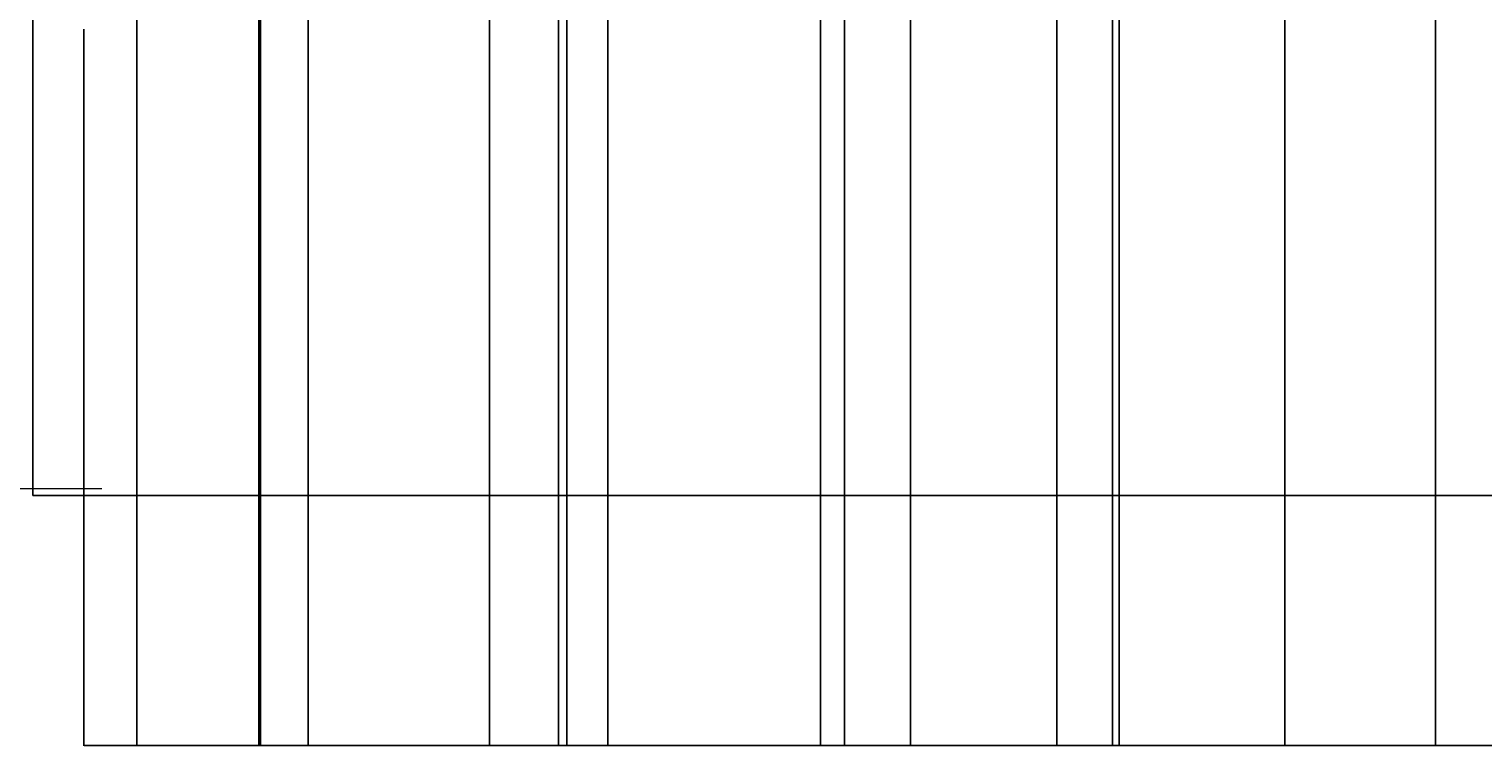
# Model space of a CAD drawing. Units: inches. Extents: x 154617 to 156384, y 250671 to 252576.
# Tile 2 of 6: x 155207 to 155945, y 250671 to 251035. Entities that reach past the tile are written whole.
import ezdxf

# ---------------------------------------------------------------- set-up
doc = ezdxf.new("R2010")
doc.units = ezdxf.units.IN
for name, color, linetype, lineweight in [('A-ANNO-DIMS', 2, 'Continuous', 18), ('C-ANNO-BRKL', 7, 'Continuous', 18), ('C-ROAD', 7, 'Continuous', 25)]:
    doc.layers.add(name, color=color, linetype=linetype, lineweight=lineweight)
doc.styles.get("Standard").update_dxf_attribs({"font": 'arial.ttf'})
doc.dimstyles.get("Standard").update_dxf_attribs({"dimtxt": 0.18, "dimasz": 0.18, "dimexe": 0.18, "dimexo": 0.0625, "dimgap": 0.09, "dimtad": 0, "dimtih": 1, "dimtoh": 1, "dimdec": 4, "dimzin": 0, "dimdsep": 46, "dimtxsty": 'Standard', "dimcen": 0.09, "dimadec": 0, "dimazin": 0, "dimtfac": 1, "dimtdec": 4, "dimtofl": 0, "dimtmove": 0, "dimatfit": 3, "dimfxl": 1, "dimtolj": 1, "dimtzin": 0, "dimarcsym": 0})

# ---------------------------------------------------------------- blocks, each defined once
blk = doc.blocks.new('ROAD-BREAK')
for p, q in [((319.88, 114.19), (261.89, 43.25)), ((319.88, 0), (319.88, 114.19)), ((261.89, 43.25), (0, 43.25)), ((344.19, 43.25), (319.88, 0)), ((540.36, 43.25), (344.19, 43.25))]:
    blk.add_line(p, q)
blk = doc.blocks.new('*D19')
at = {"layer": 'A-ANNO-DIMS', "color": 0, "lineweight": -2, "transparency": 16777216}
for p, q in [((155235.1, 251034.96), (155235.1, 250671.2)), ((156296.1, 251034.96), (156296.1, 250671.2)), ((155235.28, 250671.38), (155765.26, 250671.38)), ((156295.92, 250671.38), (155765.93, 250671.38))]:
    blk.add_line(p, q, dxfattribs=at)
at = {"layer": 'A-ANNO-DIMS', "color": 0, "transparency": 16777216}
for points in [[(155235.28, 250671.41), (155235.28, 250671.35), (155235.1, 250671.38)], [(156295.92, 250671.41), (156295.92, 250671.35), (156296.1, 250671.38)]]:
    blk.add_solid(points, dxfattribs=at)
at = {"layer": 'Defpoints', "color": 0, "transparency": 16777216}
for p in [(155235.1, 251035.03), (156296.1, 251035.03), (156296.1, 250671.38)]:
    blk.add_point(p, dxfattribs=at)
at = {"layer": 'A-ANNO-DIMS', "color": 0, "transparency": 16777216, "insert": (155765.6, 250671.38), "char_height": 0.18, "attachment_point": 5}
blk.add_mtext('\\A1;1061', dxfattribs=at)
blk = doc.blocks.new('*D24')
at = {"layer": 'A-ANNO-DIMS', "color": 0, "lineweight": -2, "transparency": 16777216}
for p, q in [((156296.16, 251035.03), (156383.38, 251035.03)), ((156383.2, 251034.85), (156383.2, 250916.83)), ((156383.2, 250798.45), (156383.2, 250916.46)), ((155209.3, 250798.27), (156383.38, 250798.27))]:
    blk.add_line(p, q, dxfattribs=at)
at = {"layer": 'A-ANNO-DIMS', "color": 0, "transparency": 16777216}
for points in [[(156383.17, 251034.85), (156383.23, 251034.85), (156383.2, 251035.03)], [(156383.17, 250798.45), (156383.23, 250798.45), (156383.2, 250798.27)]]:
    blk.add_solid(points, dxfattribs=at)
at = {"layer": 'Defpoints', "color": 0, "transparency": 16777216}
for p in [(156296.1, 251035.03), (156383.2, 251035.03), (155209.24, 250798.27)]:
    blk.add_point(p, dxfattribs=at)
at = {"layer": 'A-ANNO-DIMS', "color": 0, "transparency": 16777216, "insert": (156383.2, 250916.65), "char_height": 0.18, "attachment_point": 5}
blk.add_mtext('\\A1;236.76', dxfattribs=at)
blk = doc.blocks.new('*D36')
at = {"layer": 'A-ANNO-DIMS', "color": 0, "lineweight": -2, "transparency": 16777216}
for p, q in [((155324.84, 251443.46), (155324.84, 250671.2)), ((155475.98, 251443.46), (155475.98, 250671.2)), ((155325.02, 250671.38), (155399.96, 250671.38)), ((155475.8, 250671.38), (155400.87, 250671.38))]:
    blk.add_line(p, q, dxfattribs=at)
at = {"layer": 'A-ANNO-DIMS', "color": 0, "transparency": 16777216}
for points in [[(155325.02, 250671.41), (155325.02, 250671.35), (155324.84, 250671.38)], [(155475.8, 250671.41), (155475.8, 250671.35), (155475.98, 250671.38)]]:
    blk.add_solid(points, dxfattribs=at)
at = {"layer": 'Defpoints', "color": 0, "transparency": 16777216}
for p in [(155324.84, 251443.53), (155475.98, 251443.53), (155475.98, 250671.38)]:
    blk.add_point(p, dxfattribs=at)
at = {"layer": 'A-ANNO-DIMS', "color": 0, "transparency": 16777216, "insert": (155400.41, 250671.38), "char_height": 0.18, "attachment_point": 5}
blk.add_mtext('\\A1;151.14', dxfattribs=at)
blk = doc.blocks.new('*D37')
at = {"layer": 'A-ANNO-DIMS', "color": 0, "lineweight": -2, "transparency": 16777216}
for p, q in [((155475.98, 251443.46), (155475.98, 250671.2)), ((155654.61, 251443.46), (155654.61, 250671.2)), ((155476.16, 250671.38), (155564.84, 250671.38)), ((155654.43, 250671.38), (155565.75, 250671.38))]:
    blk.add_line(p, q, dxfattribs=at)
at = {"layer": 'A-ANNO-DIMS', "color": 0, "transparency": 16777216}
for points in [[(155476.16, 250671.41), (155476.16, 250671.35), (155475.98, 250671.38)], [(155654.43, 250671.41), (155654.43, 250671.35), (155654.61, 250671.38)]]:
    blk.add_solid(points, dxfattribs=at)
at = {"layer": 'Defpoints', "color": 0, "transparency": 16777216}
for p in [(155475.98, 251443.53), (155654.61, 251443.53), (155654.61, 250671.38)]:
    blk.add_point(p, dxfattribs=at)
at = {"layer": 'A-ANNO-DIMS', "color": 0, "transparency": 16777216, "insert": (155565.3, 250671.38), "char_height": 0.18, "attachment_point": 5}
blk.add_mtext('\\A1;178.63', dxfattribs=at)
blk = doc.blocks.new('*D38')
at = {"layer": 'A-ANNO-DIMS', "color": 0, "lineweight": -2, "transparency": 16777216}
for p, q in [((155654.61, 251443.46), (155654.61, 250671.2)), ((155757.2, 251443.46), (155757.2, 250671.2)), ((155654.79, 250671.38), (155705.45, 250671.38)), ((155757.02, 250671.38), (155706.36, 250671.38))]:
    blk.add_line(p, q, dxfattribs=at)
at = {"layer": 'A-ANNO-DIMS', "color": 0, "transparency": 16777216}
for points in [[(155654.79, 250671.41), (155654.79, 250671.35), (155654.61, 250671.38)], [(155757.02, 250671.41), (155757.02, 250671.35), (155757.2, 250671.38)]]:
    blk.add_solid(points, dxfattribs=at)
at = {"layer": 'Defpoints', "color": 0, "transparency": 16777216}
for p in [(155654.61, 251443.53), (155757.2, 251443.53), (155757.2, 250671.38)]:
    blk.add_point(p, dxfattribs=at)
at = {"layer": 'A-ANNO-DIMS', "color": 0, "transparency": 16777216, "insert": (155705.91, 250671.38), "char_height": 0.18, "attachment_point": 5}
blk.add_mtext('\\A1;102.59', dxfattribs=at)
blk = doc.blocks.new('*D39')
at = {"layer": 'A-ANNO-DIMS', "color": 0, "lineweight": -2, "transparency": 16777216}
for p, q in [((155757.2, 251443.46), (155757.2, 250671.2)), ((155844.6, 251443.46), (155844.6, 250671.2)), ((155757.38, 250671.38), (155800.58, 250671.38)), ((155844.42, 250671.38), (155801.22, 250671.38))]:
    blk.add_line(p, q, dxfattribs=at)
at = {"layer": 'A-ANNO-DIMS', "color": 0, "transparency": 16777216}
for points in [[(155757.38, 250671.41), (155757.38, 250671.35), (155757.2, 250671.38)], [(155844.42, 250671.41), (155844.42, 250671.35), (155844.6, 250671.38)]]:
    blk.add_solid(points, dxfattribs=at)
at = {"layer": 'Defpoints', "color": 0, "transparency": 16777216}
for p in [(155757.2, 251443.53), (155844.6, 251443.53), (155844.6, 250671.38)]:
    blk.add_point(p, dxfattribs=at)
at = {"layer": 'A-ANNO-DIMS', "color": 0, "transparency": 16777216, "insert": (155800.9, 250671.38), "char_height": 0.18, "attachment_point": 5}
blk.add_mtext('\\A1;87.4', dxfattribs=at)
blk = doc.blocks.new('*D40')
at = {"layer": 'A-ANNO-DIMS', "color": 0, "lineweight": -2, "transparency": 16777216}
for p, q in [((155262.1, 251119.46), (155262.1, 250671.2)), ((155324.06, 251119.46), (155324.06, 250671.2)), ((155262.28, 250671.38), (155292.69, 250671.38)), ((155323.88, 250671.38), (155293.47, 250671.38))]:
    blk.add_line(p, q, dxfattribs=at)
at = {"layer": 'A-ANNO-DIMS', "color": 0, "transparency": 16777216}
for points in [[(155262.28, 250671.41), (155262.28, 250671.35), (155262.1, 250671.38)], [(155323.88, 250671.41), (155323.88, 250671.35), (155324.06, 250671.38)]]:
    blk.add_solid(points, dxfattribs=at)
at = {"layer": 'Defpoints', "color": 0, "transparency": 16777216}
for p in [(155262.1, 251119.53), (155324.06, 251119.53), (155324.06, 250671.38)]:
    blk.add_point(p, dxfattribs=at)
at = {"layer": 'A-ANNO-DIMS', "color": 0, "transparency": 16777216, "insert": (155293.08, 250671.38), "char_height": 0.18, "attachment_point": 5}
blk.add_mtext('\\A1;61.97', dxfattribs=at)
blk = doc.blocks.new('*D52')
at = {"layer": 'A-ANNO-DIMS', "color": 0, "lineweight": -2, "transparency": 16777216}
for p, q in [((155760.6, 251155.46), (155760.6, 250671.2)), ((155844.6, 251155.46), (155844.6, 250671.2)), ((155760.78, 250671.38), (155802.38, 250671.38)), ((155844.42, 250671.38), (155802.82, 250671.38))]:
    blk.add_line(p, q, dxfattribs=at)
at = {"layer": 'A-ANNO-DIMS', "color": 0, "transparency": 16777216}
for points in [[(155760.78, 250671.41), (155760.78, 250671.35), (155760.6, 250671.38)], [(155844.42, 250671.41), (155844.42, 250671.35), (155844.6, 250671.38)]]:
    blk.add_solid(points, dxfattribs=at)
at = {"layer": 'Defpoints', "color": 0, "transparency": 16777216}
for p in [(155760.6, 251155.53), (155844.6, 251155.53), (155844.6, 250671.38)]:
    blk.add_point(p, dxfattribs=at)
at = {"layer": 'A-ANNO-DIMS', "color": 0, "transparency": 16777216, "insert": (155802.6, 250671.38), "char_height": 0.18, "attachment_point": 5}
blk.add_mtext('\\A1;84', dxfattribs=at)
blk = doc.blocks.new('*D54')
at = {"layer": 'A-ANNO-DIMS', "color": 0, "lineweight": -2, "transparency": 16777216}
for p, q in [((155844.6, 251544.74), (155844.6, 250671.2)), ((155921.1, 251544.74), (155921.1, 250671.2)), ((155844.78, 250671.38), (155882.52, 250671.38)), ((155920.92, 250671.38), (155883.17, 250671.38))]:
    blk.add_line(p, q, dxfattribs=at)
at = {"layer": 'A-ANNO-DIMS', "color": 0, "transparency": 16777216}
for points in [[(155844.78, 250671.41), (155844.78, 250671.35), (155844.6, 250671.38)], [(155920.92, 250671.41), (155920.92, 250671.35), (155921.1, 250671.38)]]:
    blk.add_solid(points, dxfattribs=at)
at = {"layer": 'Defpoints', "color": 0, "transparency": 16777216}
for p in [(155844.6, 251544.8), (155921.1, 251544.8), (155921.1, 250671.38)]:
    blk.add_point(p, dxfattribs=at)
at = {"layer": 'A-ANNO-DIMS', "color": 0, "transparency": 16777216, "insert": (155882.85, 250671.38), "char_height": 0.18, "attachment_point": 5}
blk.add_mtext('\\A1;76.5', dxfattribs=at)
blk = doc.blocks.new('*D56')
at = {"layer": 'A-ANNO-DIMS', "color": 0, "lineweight": -2, "transparency": 16777216}
for p, q in [((155324.06, 251119.46), (155324.06, 250671.2)), ((155480.24, 251119.46), (155480.24, 250671.2)), ((155324.24, 250671.38), (155401.7, 250671.38)), ((155480.06, 250671.38), (155402.61, 250671.38))]:
    blk.add_line(p, q, dxfattribs=at)
at = {"layer": 'A-ANNO-DIMS', "color": 0, "transparency": 16777216}
for points in [[(155324.24, 250671.41), (155324.24, 250671.35), (155324.06, 250671.38)], [(155480.06, 250671.41), (155480.06, 250671.35), (155480.24, 250671.38)]]:
    blk.add_solid(points, dxfattribs=at)
at = {"layer": 'Defpoints', "color": 0, "transparency": 16777216}
for p in [(155324.06, 251119.53), (155480.24, 251119.53), (155480.24, 250671.38)]:
    blk.add_point(p, dxfattribs=at)
at = {"layer": 'A-ANNO-DIMS', "color": 0, "transparency": 16777216, "insert": (155402.15, 250671.38), "char_height": 0.18, "attachment_point": 5}
blk.add_mtext('\\A1;156.18', dxfattribs=at)
blk = doc.blocks.new('*D57')
at = {"layer": 'A-ANNO-DIMS', "color": 0, "lineweight": -2, "transparency": 16777216}
for p, q in [((155480.24, 251119.46), (155480.24, 250671.2)), ((155608.93, 251119.46), (155608.93, 250671.2)), ((155480.42, 250671.38), (155544.13, 250671.38)), ((155608.75, 250671.38), (155545.04, 250671.38))]:
    blk.add_line(p, q, dxfattribs=at)
at = {"layer": 'A-ANNO-DIMS', "color": 0, "transparency": 16777216}
for points in [[(155480.42, 250671.41), (155480.42, 250671.35), (155480.24, 250671.38)], [(155608.75, 250671.41), (155608.75, 250671.35), (155608.93, 250671.38)]]:
    blk.add_solid(points, dxfattribs=at)
at = {"layer": 'Defpoints', "color": 0, "transparency": 16777216}
for p in [(155480.24, 251119.53), (155608.93, 251119.53), (155608.93, 250671.38)]:
    blk.add_point(p, dxfattribs=at)
at = {"layer": 'A-ANNO-DIMS', "color": 0, "transparency": 16777216, "insert": (155544.58, 250671.38), "char_height": 0.18, "attachment_point": 5}
blk.add_mtext('\\A1;128.68', dxfattribs=at)
blk = doc.blocks.new('*D59')
at = {"layer": 'A-ANNO-DIMS', "color": 0, "lineweight": -2, "transparency": 16777216}
for p, q in [((155348.98, 251598.96), (155348.98, 250671.2)), ((155441.1, 251598.96), (155441.1, 250671.2)), ((155349.16, 250671.38), (155394.65, 250671.38)), ((155440.92, 250671.38), (155395.43, 250671.38))]:
    blk.add_line(p, q, dxfattribs=at)
at = {"layer": 'A-ANNO-DIMS', "color": 0, "transparency": 16777216}
for points in [[(155349.16, 250671.41), (155349.16, 250671.35), (155348.98, 250671.38)], [(155440.92, 250671.41), (155440.92, 250671.35), (155441.1, 250671.38)]]:
    blk.add_solid(points, dxfattribs=at)
at = {"layer": 'Defpoints', "color": 0, "transparency": 16777216}
for p in [(155348.98, 251599.03), (155441.1, 251599.03), (155441.1, 250671.38)]:
    blk.add_point(p, dxfattribs=at)
at = {"layer": 'A-ANNO-DIMS', "color": 0, "transparency": 16777216, "insert": (155395.04, 250671.38), "char_height": 0.18, "attachment_point": 5}
blk.add_mtext('\\A1;92.12', dxfattribs=at)
blk = doc.blocks.new('*D60')
at = {"layer": 'A-ANNO-DIMS', "color": 0, "lineweight": -2, "transparency": 16777216}
for p, q in [((155441.1, 251598.96), (155441.1, 250671.2)), ((155501.1, 251598.96), (155501.1, 250671.2)), ((155441.28, 250671.38), (155470.88, 250671.38)), ((155500.92, 250671.38), (155471.32, 250671.38))]:
    blk.add_line(p, q, dxfattribs=at)
at = {"layer": 'A-ANNO-DIMS', "color": 0, "transparency": 16777216}
for points in [[(155441.28, 250671.41), (155441.28, 250671.35), (155441.1, 250671.38)], [(155500.92, 250671.41), (155500.92, 250671.35), (155501.1, 250671.38)]]:
    blk.add_solid(points, dxfattribs=at)
at = {"layer": 'Defpoints', "color": 0, "transparency": 16777216}
for p in [(155441.1, 251599.03), (155501.1, 251599.03), (155501.1, 250671.38)]:
    blk.add_point(p, dxfattribs=at)
at = {"layer": 'A-ANNO-DIMS', "color": 0, "transparency": 16777216, "insert": (155471.1, 250671.38), "char_height": 0.18, "attachment_point": 5}
blk.add_mtext('\\A1;60', dxfattribs=at)
blk = doc.blocks.new('*D61')
at = {"layer": 'A-ANNO-DIMS', "color": 0, "lineweight": -2, "transparency": 16777216}
for p, q in [((155501.1, 251598.96), (155501.1, 250671.2)), ((155621.1, 251598.96), (155621.1, 250671.2)), ((155501.28, 250671.38), (155560.82, 250671.38)), ((155620.92, 250671.38), (155561.38, 250671.38))]:
    blk.add_line(p, q, dxfattribs=at)
at = {"layer": 'A-ANNO-DIMS', "color": 0, "transparency": 16777216}
for points in [[(155501.28, 250671.41), (155501.28, 250671.35), (155501.1, 250671.38)], [(155620.92, 250671.41), (155620.92, 250671.35), (155621.1, 250671.38)]]:
    blk.add_solid(points, dxfattribs=at)
at = {"layer": 'Defpoints', "color": 0, "transparency": 16777216}
for p in [(155501.1, 251599.03), (155621.1, 251599.03), (155621.1, 250671.38)]:
    blk.add_point(p, dxfattribs=at)
at = {"layer": 'A-ANNO-DIMS', "color": 0, "transparency": 16777216, "insert": (155561.1, 250671.38), "char_height": 0.18, "attachment_point": 5}
blk.add_mtext('\\A1;120', dxfattribs=at)
blk = doc.blocks.new('*D68')
at = {"layer": 'A-ANNO-DIMS', "color": 0, "lineweight": -2, "transparency": 16777216}
for p, q in [((155760.6, 251155.46), (155760.6, 250671.2)), ((155728.93, 251119.46), (155728.93, 250671.2)), ((155729.11, 250671.38), (155744.37, 250671.38)), ((155760.42, 250671.38), (155745.16, 250671.38))]:
    blk.add_line(p, q, dxfattribs=at)
at = {"layer": 'A-ANNO-DIMS', "color": 0, "transparency": 16777216}
for points in [[(155729.11, 250671.41), (155729.11, 250671.35), (155728.93, 250671.38)], [(155760.42, 250671.41), (155760.42, 250671.35), (155760.6, 250671.38)]]:
    blk.add_solid(points, dxfattribs=at)
at = {"layer": 'Defpoints', "color": 0, "transparency": 16777216}
for p in [(155760.6, 251155.53), (155728.93, 251119.53), (155760.6, 250671.38)]:
    blk.add_point(p, dxfattribs=at)
at = {"layer": 'A-ANNO-DIMS', "color": 0, "transparency": 16777216, "insert": (155744.76, 250671.38), "char_height": 0.18, "attachment_point": 5}
blk.add_mtext('\\A1;31.67', dxfattribs=at)

msp = doc.modelspace()

# ---------------------------------------------------------------- linework, layer by layer
at = {"layer": 'C-ROAD'}
msp.add_line((155209.237, 252414.495), (155209.237, 250798.266), dxfattribs=at)

# ---------------------------------------------------------------- block references
at = {"layer": 'C-ANNO-BRKL'}
msp.add_blockref('ROAD-BREAK', (154704.015, 250758.479), dxfattribs=at)

# ---------------------------------------------------------------- dimensions: what is measured, and where the dimension line sits
at = {"layer": 'A-ANNO-DIMS'}
for base, p1, p2, override, picture, middle in [((155441.0971, 250671.3791), (155348.9817, 251599.0264), (155441.0971, 251599.0264), {"dimdec": 2, "dimlfac": 1, "dimrnd": 0, "dimzin": 0, "dimdsep": 46, "dimlunit": 2}, '*D59', (155395.0394, 250671.3791)), ((155501.097, 250671.379), (155441.097, 251599.026), (155501.097, 251599.026), {"dimdec": 0, "dimlfac": 1, "dimrnd": 0, "dimzin": 0, "dimdsep": 46, "dimlunit": 2}, '*D60', (155471.097, 250671.379)), ((155621.097, 250671.379), (155501.097, 251599.026), (155621.097, 251599.026), {"dimdec": 0, "dimlfac": 1, "dimrnd": 0, "dimzin": 0, "dimdsep": 46, "dimlunit": 2}, '*D61', (155561.097, 250671.379)), ((155921.097, 250671.379), (155844.597, 251544.802), (155921.097, 251544.802), {"dimdec": 1, "dimlfac": 1, "dimrnd": 0, "dimzin": 0, "dimdsep": 46, "dimlunit": 2}, '*D54', (155882.847, 250671.379)), ((155475.98, 250671.379), (155324.842, 251443.526), (155475.98, 251443.526), {"dimdec": 2, "dimlfac": 1, "dimrnd": 0, "dimzin": 0, "dimdsep": 46, "dimlunit": 2}, '*D36', (155400.411, 250671.379)), ((155654.613, 250671.379), (155475.98, 251443.526), (155654.613, 251443.526), {"dimdec": 2, "dimlfac": 1, "dimrnd": 0, "dimzin": 0, "dimdsep": 46, "dimlunit": 2}, '*D37', (155565.297, 250671.379)), ((155757.203, 250671.379), (155654.613, 251443.526), (155757.203, 251443.526), {"dimdec": 2, "dimlfac": 1, "dimrnd": 0, "dimzin": 0, "dimdsep": 46, "dimlunit": 2}, '*D38', (155705.908, 250671.379)), ((155844.597, 250671.379), (155757.203, 251443.526), (155844.597, 251443.526), {"dimdec": 1, "dimlfac": 1, "dimrnd": 0, "dimzin": 0, "dimdsep": 46, "dimlunit": 2}, '*D39', (155800.9, 250671.379)), ((155760.597, 250671.379), (155728.926, 251119.526), (155760.597, 251155.526), {"dimdec": 2, "dimlfac": 1, "dimrnd": 0, "dimzin": 0, "dimdsep": 46, "dimlunit": 2}, '*D68', (155744.761, 250671.379)), ((155844.597, 250671.379), (155760.597, 251155.526), (155844.597, 251155.526), {"dimdec": 0, "dimlfac": 1, "dimrnd": 0, "dimzin": 0, "dimdsep": 46, "dimlunit": 2}, '*D52', (155802.597, 250671.379)), ((155324.063, 250671.379), (155262.097, 251119.526), (155324.063, 251119.526), {"dimdec": 2, "dimlfac": 1, "dimrnd": 0, "dimzin": 0, "dimdsep": 46, "dimlunit": 2}, '*D40', (155293.08, 250671.379)), ((155480.244, 250671.379), (155324.063, 251119.526), (155480.244, 251119.526), {"dimdec": 2, "dimlfac": 1, "dimrnd": 0, "dimzin": 0, "dimdsep": 46, "dimlunit": 2}, '*D56', (155402.154, 250671.379)), ((155608.926, 250671.379), (155480.244, 251119.526), (155608.926, 251119.526), {"dimdec": 2, "dimlfac": 1, "dimrnd": 0, "dimzin": 0, "dimdsep": 46, "dimlunit": 2}, '*D57', (155544.585, 250671.379)), ((156296.097, 250671.379), (155235.097, 251035.026), (156296.097, 251035.026), {"dimdec": 0, "dimlfac": 1, "dimrnd": 0, "dimzin": 0, "dimdsep": 46, "dimlunit": 2}, '*D19', (155765.597, 250671.379))]:
    dim = msp.add_linear_dim(base=base, p1=p1, p2=p2, dimstyle='Standard', override=override, dxfattribs=at)
    dim.commit()
    dim.dimension.update_dxf_attribs({"geometry": picture, "text_midpoint": middle})
dim = msp.add_linear_dim(base=(156383.197, 251035.026), p1=(155209.237, 250798.266), p2=(156296.097, 251035.026), angle=90, dimstyle='Standard', override={"dimdec": 2, "dimlfac": 1, "dimrnd": 0, "dimzin": 0, "dimdsep": 46, "dimlunit": 2}, dxfattribs=at)
dim.commit()
dim.dimension.update_dxf_attribs({"geometry": '*D24', "text_midpoint": (156383.197, 250916.646)})

doc.saveas('drawing.dxf')
